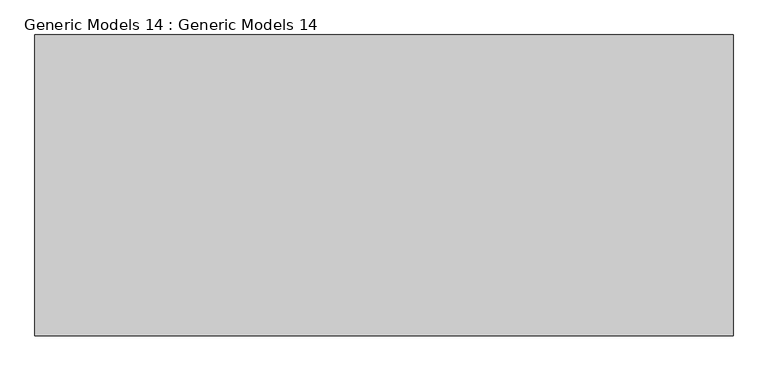
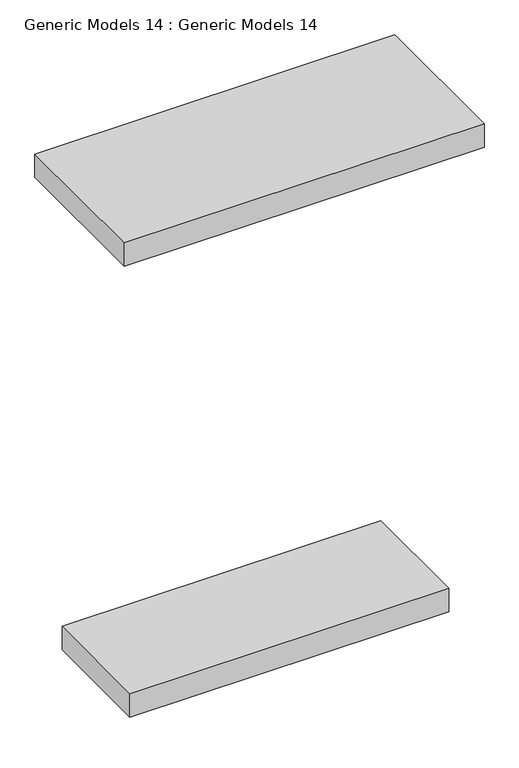
"""IFC4 building model written with IfcOpenShell, lengths in millimetres: proxy geometry, Generic Models 14 : Generic Models 14."""

from ifc_helpers import new_model, si_unit, frame, origin, place, context, project, spatial, polyline, outline, extrude, source, transform, mapped, element, save


def generic_models_14_generic_models_14_0d0b8766(model_context):
    return source(origin(), model_context, "Body", "SweptSolid", [
        extrude(outline(polyline([(-11823.5341583, 3667.5222768), (-11823.5341583, 4389.2432846), (-9860.3859258, 4389.2432846), (-9860.3859258, 3667.5222768), (-11823.5341583, 3667.5222768)])), frame((0.0, 0.0, 2530.5665304), z_axis=(0.0, 0.0, 1.0), x_axis=(1.0, 0.0, 0.0)), (0.0, 0.0, 1.0), 152.4),
        extrude(outline(polyline([(-11923.2597985, 3553.2222768), (-11923.2597985, 4507.5695976), (-9707.9859258, 4507.5695976), (-9707.9859258, 3553.2222768), (-11923.2597985, 3553.2222768)])), frame((0.0, 0.0, 5569.8192996), z_axis=(0.0, 0.0, 1.0), x_axis=(1.0, 0.0, 0.0)), (0.0, 0.0, 1.0), 152.4),
    ])


if __name__ == "__main__":
    model = new_model("IFC4")
    model_context = context("Model", 3, world=origin())
    ifc_project = project(units=[si_unit("LENGTHUNIT", "METRE", prefix="MILLI")], contexts=[model_context])
    site = spatial("IfcSite", under=ifc_project)
    building = spatial("IfcBuilding", under=site)
    placement = place(None, origin())
    generic_models_14_generic_models_14_shape = generic_models_14_generic_models_14_0d0b8766(model_context)
    element("IfcBuildingElementProxy", 1, Name="Generic Models 14 : Generic Models 14", ObjectType="Generic Models 14 : Generic Models 14", at=placement, inside=building, context=model_context, shape_type="MappedRepresentation", body=[
        mapped(generic_models_14_generic_models_14_shape, transform((0.0, 0.0, 0.0), x_axis=(1.0, 0.0, 0.0), y_axis=(0.0, 1.0, 0.0), z_axis=(0.0, 0.0, 1.0))),
    ])
    save(model, "model.ifc")
